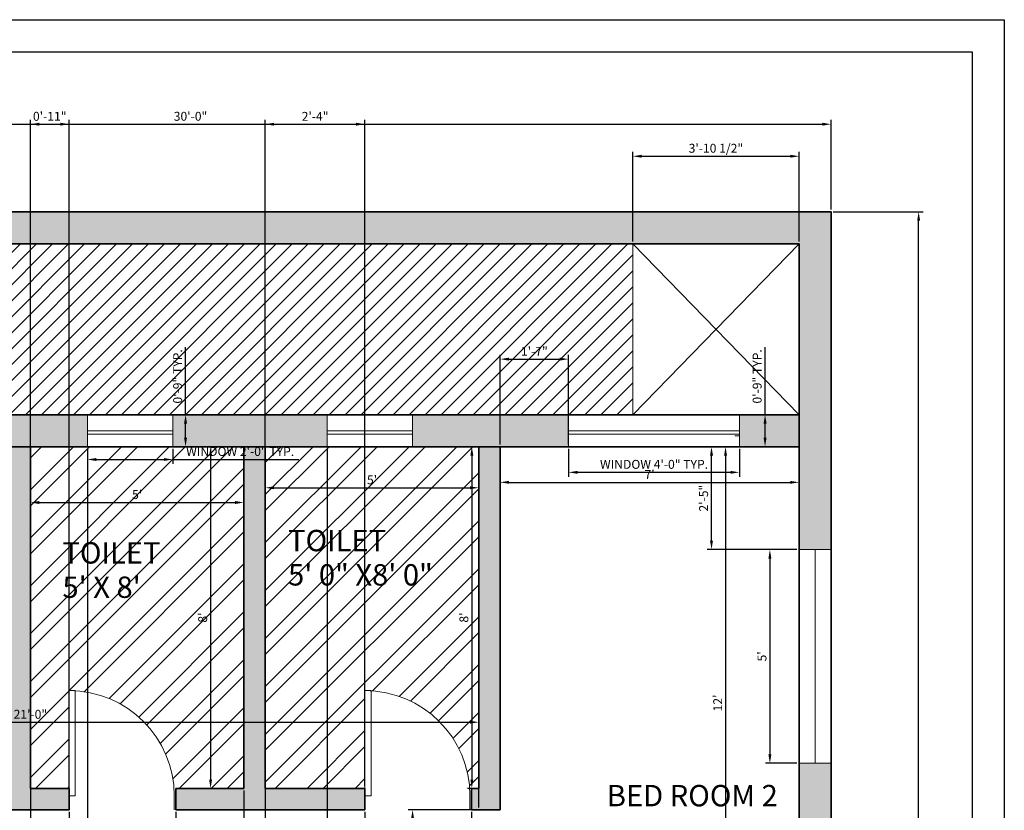
# Model space of a CAD drawing. Units: inches. Extents: x 2998 to 3448, y 1620 to 2377.
# Tile 5 of 5: x 3171 to 3448, y 2155 to 2377. Entities that reach past the tile are written whole.
import ezdxf

# ---------------------------------------------------------------- set-up
doc = ezdxf.new("R2010")
doc.units = ezdxf.units.IN
doc.layers.get('Defpoints').update_dxf_attribs({"color": 110})
for name, color, linetype, lineweight in [('A-ANNO-DIMS', 2, 'Continuous', 18), ('A-ANNO-TTLB', 7, 'Continuous', 25), ('A-AREA-IDEN', 130, 'Continuous', 18), ('A-DOOR', 3, 'Continuous', 18), ('A-FLOR-OPEN', 7, 'Continuous', 18), ('A-FLOR-PATT', 18, 'Continuous', 13), ('A-GLAZ', 4, 'Continuous', 18), ('A-WALL-PATT', 18, 'Continuous', 13), ('C-PROP', 7, 'Continuous', 35), ('L-HRDS-PATT', 175, 'Continuous', 13), ('WALL', 7, 'Continuous', 35)]:
    doc.layers.add(name, color=color, linetype=linetype, lineweight=lineweight)
doc.styles.get("Standard").update_dxf_attribs({"font": 'arial.ttf'})
doc.dimstyles.new('Copy of ISO-25', dxfattribs={"dimtxt": 2.5, "dimasz": 2.5, "dimexe": 1.25, "dimexo": 0.625, "dimtad": 1, "dimdec": 1, "dimlunit": 4, "dimtxsty": 'Standard', "dimcen": 2.5, "dimadec": 0, "dimazin": 0, "dimtfac": 1, "dimtdec": 1, "dimtmove": 0, "dimatfit": 3, "dimfxl": 1, "dimarcsym": 0})

# ---------------------------------------------------------------- blocks, each defined once
blk = doc.blocks.new('*U2')
for p, q in [((0, 0), (0, -100)), ((750, 0), (750, -100))]:
    blk.add_line(p, q)
blk.add_lwpolyline([(0, 0), (0, 750), (43.75, 750), (43.75, 0)], close=True)
blk.add_arc((0, 0), 750, 0, 90)
blk = doc.blocks.new('*D8')
at = {"layer": 'A-ANNO-DIMS', "color": 0, "lineweight": -2, "transparency": 16777216}
for p, q in [((3174.12, 2256.15), (3174.12, 2239.84)), ((3234.12, 2256.15), (3234.12, 2239.84)), ((3176.62, 2241.09), (3231.62, 2241.09))]:
    blk.add_line(p, q, dxfattribs=at)
at = {"layer": 'A-ANNO-DIMS', "color": 0, "transparency": 16777216}
for points in [[(3176.62, 2241.51), (3176.62, 2240.68), (3174.12, 2241.09)], [(3231.62, 2241.51), (3231.62, 2240.68), (3234.12, 2241.09)]]:
    blk.add_solid(points, dxfattribs=at)
at = {"layer": 'Defpoints', "color": 0, "transparency": 16777216}
for p in [(3174.12, 2256.77), (3234.12, 2256.77), (3234.12, 2241.09)]:
    blk.add_point(p, dxfattribs=at)
at = {"layer": 'A-ANNO-DIMS', "color": 0, "transparency": 16777216, "insert": (3204.12, 2242.99), "char_height": 2.5, "attachment_point": 5}
blk.add_mtext("5'", dxfattribs=at)
blk = doc.blocks.new('*D9')
at = {"layer": 'A-ANNO-DIMS', "color": 0, "lineweight": -2, "transparency": 16777216}
for p, q in [((3233.49, 2256.77), (3223.51, 2256.77)), ((3224.76, 2254.27), (3224.76, 2163.27)), ((3233.49, 2160.77), (3223.51, 2160.77))]:
    blk.add_line(p, q, dxfattribs=at)
at = {"layer": 'A-ANNO-DIMS', "color": 0, "transparency": 16777216}
for points in [[(3224.34, 2254.27), (3225.18, 2254.27), (3224.76, 2256.77)], [(3224.34, 2163.27), (3225.18, 2163.27), (3224.76, 2160.77)]]:
    blk.add_solid(points, dxfattribs=at)
at = {"layer": 'Defpoints', "color": 0, "transparency": 16777216}
for p in [(3234.12, 2256.77), (3224.76, 2160.77), (3234.12, 2160.77)]:
    blk.add_point(p, dxfattribs=at)
at = {"layer": 'A-ANNO-DIMS', "color": 0, "transparency": 16777216, "insert": (3222.86, 2208.77), "char_height": 2.5, "attachment_point": 5, "rotation": 90}
blk.add_mtext("8'", dxfattribs=at)
blk = doc.blocks.new('*D10')
at = {"layer": 'A-ANNO-DIMS', "color": 0, "lineweight": -2, "transparency": 16777216}
for p, q in [((3240.12, 2256.15), (3240.12, 2243.98)), ((3300.12, 2256.15), (3300.12, 2243.98)), ((3242.62, 2245.23), (3297.62, 2245.23))]:
    blk.add_line(p, q, dxfattribs=at)
at = {"layer": 'A-ANNO-DIMS', "color": 0, "transparency": 16777216}
for points in [[(3242.62, 2245.65), (3242.62, 2244.82), (3240.12, 2245.23)], [(3297.62, 2245.65), (3297.62, 2244.82), (3300.12, 2245.23)]]:
    blk.add_solid(points, dxfattribs=at)
at = {"layer": 'Defpoints', "color": 0, "transparency": 16777216}
for p in [(3240.12, 2256.77), (3300.12, 2256.77), (3300.12, 2245.23)]:
    blk.add_point(p, dxfattribs=at)
at = {"layer": 'A-ANNO-DIMS', "color": 0, "transparency": 16777216, "insert": (3270.12, 2247.13), "char_height": 2.5, "attachment_point": 5}
blk.add_mtext("5'", dxfattribs=at)
blk = doc.blocks.new('*D11')
at = {"layer": 'A-ANNO-DIMS', "color": 0, "lineweight": -2, "transparency": 16777216}
for p, q in [((3299.49, 2256.77), (3296.92, 2256.77)), ((3298.17, 2254.27), (3298.17, 2163.27)), ((3299.49, 2160.77), (3296.92, 2160.77))]:
    blk.add_line(p, q, dxfattribs=at)
at = {"layer": 'A-ANNO-DIMS', "color": 0, "transparency": 16777216}
for points in [[(3297.75, 2254.27), (3298.58, 2254.27), (3298.17, 2256.77)], [(3297.75, 2163.27), (3298.58, 2163.27), (3298.17, 2160.77)]]:
    blk.add_solid(points, dxfattribs=at)
at = {"layer": 'Defpoints', "color": 0, "transparency": 16777216}
for p in [(3300.12, 2256.77), (3298.17, 2160.77), (3300.12, 2160.77)]:
    blk.add_point(p, dxfattribs=at)
at = {"layer": 'A-ANNO-DIMS', "color": 0, "transparency": 16777216, "insert": (3296.26, 2208.77), "char_height": 2.5, "attachment_point": 5, "rotation": 90}
blk.add_mtext("8'", dxfattribs=at)
blk = doc.blocks.new('*D12')
at = {"layer": 'A-ANNO-DIMS', "color": 0, "lineweight": -2, "transparency": 16777216}
for p, q in [((3306.12, 2256.15), (3306.12, 2245.51)), ((3390.12, 2256.15), (3390.12, 2245.51)), ((3308.62, 2246.76), (3387.62, 2246.76))]:
    blk.add_line(p, q, dxfattribs=at)
at = {"layer": 'A-ANNO-DIMS', "color": 0, "transparency": 16777216}
for points in [[(3308.62, 2247.18), (3308.62, 2246.35), (3306.12, 2246.76)], [(3387.62, 2247.18), (3387.62, 2246.35), (3390.12, 2246.76)]]:
    blk.add_solid(points, dxfattribs=at)
at = {"layer": 'Defpoints', "color": 0, "transparency": 16777216}
for p in [(3306.12, 2256.77), (3390.12, 2256.77), (3390.12, 2246.76)]:
    blk.add_point(p, dxfattribs=at)
at = {"layer": 'A-ANNO-DIMS', "color": 0, "transparency": 16777216, "insert": (3348.12, 2248.64), "char_height": 2.5, "attachment_point": 5}
blk.add_mtext("7'", dxfattribs=at)
blk = doc.blocks.new('*D13')
at = {"layer": 'A-ANNO-DIMS', "color": 0, "lineweight": -2, "transparency": 16777216}
for p, q in [((3389.49, 2256.77), (3368.21, 2256.77)), ((3369.46, 2254.27), (3369.46, 2115.27)), ((3389.49, 2112.77), (3368.21, 2112.77))]:
    blk.add_line(p, q, dxfattribs=at)
at = {"layer": 'A-ANNO-DIMS', "color": 0, "transparency": 16777216}
for points in [[(3369.04, 2254.27), (3369.87, 2254.27), (3369.46, 2256.77)], [(3369.04, 2115.27), (3369.87, 2115.27), (3369.46, 2112.77)]]:
    blk.add_solid(points, dxfattribs=at)
at = {"layer": 'Defpoints', "color": 0, "transparency": 16777216}
for p in [(3390.12, 2256.77), (3369.46, 2112.77), (3390.12, 2112.77)]:
    blk.add_point(p, dxfattribs=at)
at = {"layer": 'A-ANNO-DIMS', "color": 0, "transparency": 16777216, "insert": (3367.58, 2184.77), "char_height": 2.5, "attachment_point": 5, "rotation": 90}
blk.add_mtext("12'", dxfattribs=at)
blk = doc.blocks.new('*D23')
at = {"layer": 'A-ANNO-DIMS', "color": 0, "lineweight": -2, "transparency": 16777216}
for p, q in [((3389.49, 2227.86), (3380.67, 2227.86)), ((3381.92, 2225.36), (3381.92, 2170.36)), ((3389.49, 2167.86), (3380.67, 2167.86))]:
    blk.add_line(p, q, dxfattribs=at)
at = {"layer": 'A-ANNO-DIMS', "color": 0, "transparency": 16777216}
for points in [[(3381.5, 2225.36), (3382.34, 2225.36), (3381.92, 2227.86)], [(3381.5, 2170.36), (3382.34, 2170.36), (3381.92, 2167.86)]]:
    blk.add_solid(points, dxfattribs=at)
at = {"layer": 'Defpoints', "color": 0, "transparency": 16777216}
for p in [(3390.12, 2227.86), (3381.92, 2167.86), (3390.12, 2167.86)]:
    blk.add_point(p, dxfattribs=at)
at = {"layer": 'A-ANNO-DIMS', "color": 0, "transparency": 16777216, "insert": (3380.02, 2197.86), "char_height": 2.5, "attachment_point": 5, "rotation": 90}
blk.add_mtext("5'", dxfattribs=at)
blk = doc.blocks.new('WIN-24IN')
for p, q in [((0, 0), (0, 9)), ((0, 9), (24, 9)), ((24, 9), (24, 0)), ((0, 4.5), (24, 4.5)), ((0, 3.5), (24, 3.5))]:
    blk.add_line(p, q)
blk = doc.blocks.new('WIN-48IN')
for p, q in [((0, 0), (0, 9)), ((0, 9), (48, 9)), ((48, 9), (48, 0)), ((0, 4.5), (48, 4.5)), ((0, 3.5), (48, 3.5))]:
    blk.add_line(p, q)
blk = doc.blocks.new('*D31')
at = {"layer": 'A-ANNO-DIMS', "color": 0, "lineweight": -2, "transparency": 16777216}
for p, q in [((3325.36, 2256.15), (3325.36, 2248.32)), ((3373.36, 2256.15), (3373.36, 2248.32)), ((3327.86, 2249.57), (3370.86, 2249.57))]:
    blk.add_line(p, q, dxfattribs=at)
at = {"layer": 'A-ANNO-DIMS', "color": 0, "transparency": 16777216}
for points in [[(3327.86, 2249.99), (3327.86, 2249.16), (3325.36, 2249.57)], [(3370.86, 2249.99), (3370.86, 2249.16), (3373.36, 2249.57)]]:
    blk.add_solid(points, dxfattribs=at)
at = {"layer": 'Defpoints', "color": 0}
for p in [(3325.36, 2256.77), (3373.36, 2256.77), (3373.36, 2249.57)]:
    blk.add_point(p, dxfattribs=at)
at = {"layer": 'A-ANNO-DIMS', "color": 0, "transparency": 16777216, "insert": (3349.36, 2251.49), "char_height": 2.5, "attachment_point": 5}
blk.add_mtext('WINDOW 4\'-0" TYP.', dxfattribs=at)
blk = doc.blocks.new('*D32')
at = {"layer": 'A-ANNO-DIMS', "color": 0, "lineweight": -2, "transparency": 16777216}
for p, q in [((3380.56, 2265.77), (3380.56, 2284.76)), ((3373.99, 2265.77), (3381.81, 2265.77)), ((3380.56, 2259.27), (3380.56, 2263.27)), ((3373.99, 2256.77), (3381.81, 2256.77))]:
    blk.add_line(p, q, dxfattribs=at)
at = {"layer": 'A-ANNO-DIMS', "color": 0, "transparency": 16777216}
for points in [[(3380.15, 2263.27), (3380.98, 2263.27), (3380.56, 2265.77)], [(3380.15, 2259.27), (3380.98, 2259.27), (3380.56, 2256.77)]]:
    blk.add_solid(points, dxfattribs=at)
at = {"layer": 'Defpoints', "color": 0}
for p in [(3373.36, 2265.77), (3380.56, 2265.77), (3373.36, 2256.77)]:
    blk.add_point(p, dxfattribs=at)
at = {"layer": 'A-ANNO-DIMS', "color": 0, "transparency": 16777216, "insert": (3378.66, 2276.52), "char_height": 2.5, "attachment_point": 5, "rotation": 90}
blk.add_mtext('0\'-9" TYP.', dxfattribs=at)
blk = doc.blocks.new('*D33')
at = {"layer": 'A-ANNO-DIMS', "color": 0, "lineweight": -2, "transparency": 16777216}
for p, q in [((3190.13, 2256.15), (3190.13, 2251.92)), ((3214.13, 2256.15), (3214.13, 2251.92)), ((3192.63, 2253.17), (3211.63, 2253.17)), ((3214.13, 2253.17), (3249.51, 2253.17))]:
    blk.add_line(p, q, dxfattribs=at)
at = {"layer": 'A-ANNO-DIMS', "color": 0, "transparency": 16777216}
for points in [[(3192.63, 2253.59), (3192.63, 2252.76), (3190.13, 2253.17)], [(3211.63, 2253.59), (3211.63, 2252.76), (3214.13, 2253.17)]]:
    blk.add_solid(points, dxfattribs=at)
at = {"layer": 'Defpoints', "color": 0}
for p in [(3190.13, 2256.77), (3214.13, 2256.77), (3214.13, 2253.17)]:
    blk.add_point(p, dxfattribs=at)
at = {"layer": 'A-ANNO-DIMS', "color": 0, "transparency": 16777216, "insert": (3233.07, 2255.09), "char_height": 2.5, "attachment_point": 5}
blk.add_mtext('WINDOW 2\'-0" TYP.', dxfattribs=at)
blk = doc.blocks.new('*D34')
at = {"layer": 'A-ANNO-DIMS', "color": 0, "lineweight": -2, "transparency": 16777216}
for p, q in [((3217.73, 2265.77), (3217.73, 2284.76)), ((3214.75, 2265.77), (3218.98, 2265.77)), ((3217.73, 2259.27), (3217.73, 2263.27)), ((3214.75, 2256.77), (3218.98, 2256.77))]:
    blk.add_line(p, q, dxfattribs=at)
at = {"layer": 'A-ANNO-DIMS', "color": 0, "transparency": 16777216}
for points in [[(3217.31, 2263.27), (3218.14, 2263.27), (3217.73, 2265.77)], [(3217.31, 2259.27), (3218.14, 2259.27), (3217.73, 2256.77)]]:
    blk.add_solid(points, dxfattribs=at)
at = {"layer": 'Defpoints', "color": 0}
for p in [(3214.13, 2265.77), (3217.73, 2265.77), (3214.13, 2256.77)]:
    blk.add_point(p, dxfattribs=at)
at = {"layer": 'A-ANNO-DIMS', "color": 0, "transparency": 16777216, "insert": (3215.83, 2276.52), "char_height": 2.5, "attachment_point": 5, "rotation": 90}
blk.add_mtext('0\'-9" TYP.', dxfattribs=at)
blk = doc.blocks.new('*D39')
at = {"layer": 'A-ANNO-DIMS', "color": 0, "lineweight": -2, "transparency": 16777216}
for p, q in [((3039.12, 2323.4), (3039.12, 2348.62)), ((3041.62, 2347.37), (3396.62, 2347.37)), ((3399.12, 2323.4), (3399.12, 2348.62))]:
    blk.add_line(p, q, dxfattribs=at)
at = {"layer": 'A-ANNO-DIMS', "color": 0, "transparency": 16777216}
for points in [[(3041.62, 2347.79), (3041.62, 2346.96), (3039.12, 2347.37)], [(3396.62, 2347.79), (3396.62, 2346.96), (3399.12, 2347.37)]]:
    blk.add_solid(points, dxfattribs=at)
at = {"layer": 'Defpoints', "color": 0}
for p in [(3399.12, 2347.37), (3039.12, 2322.77), (3399.12, 2322.77)]:
    blk.add_point(p, dxfattribs=at)
at = {"layer": 'A-ANNO-DIMS', "color": 0, "transparency": 16777216, "insert": (3219.12, 2349.27), "char_height": 2.5, "attachment_point": 5}
blk.add_mtext('30\'-0"', dxfattribs=at)
blk = doc.blocks.new('*D40')
at = {"layer": 'A-ANNO-DIMS', "color": 0, "lineweight": -2, "transparency": 16777216}
for p, q in [((3399.74, 2322.77), (3424.97, 2322.77)), ((3423.72, 1845.27), (3423.72, 2320.27)), ((3399.74, 1842.77), (3424.97, 1842.77))]:
    blk.add_line(p, q, dxfattribs=at)
at = {"layer": 'A-ANNO-DIMS', "color": 0, "transparency": 16777216}
for points in [[(3423.3, 2320.27), (3424.14, 2320.27), (3423.72, 2322.77)], [(3423.3, 1845.27), (3424.14, 1845.27), (3423.72, 1842.77)]]:
    blk.add_solid(points, dxfattribs=at)
at = {"layer": 'Defpoints', "color": 0}
for p in [(3399.12, 2322.77), (3423.72, 2322.77), (3399.12, 1842.77)]:
    blk.add_point(p, dxfattribs=at)
at = {"layer": 'A-ANNO-DIMS', "color": 0, "transparency": 16777216, "insert": (3421.82, 2082.77), "char_height": 2.5, "attachment_point": 5, "rotation": 90}
blk.add_mtext('40\'-0"', dxfattribs=at)
blk = doc.blocks.new('*D51')
at = {"layer": 'A-ANNO-DIMS', "color": 0, "lineweight": -2, "transparency": 16777216}
for p, q in [((3174.12, 2256.15), (3174.12, 1816.92)), ((3190.13, 2256.15), (3190.13, 1816.92)), ((3176.62, 1818.17), (3187.63, 1818.17))]:
    blk.add_line(p, q, dxfattribs=at)
at = {"layer": 'A-ANNO-DIMS', "color": 0, "transparency": 16777216}
for points in [[(3176.62, 1818.59), (3176.62, 1817.76), (3174.12, 1818.17)], [(3187.63, 1818.59), (3187.63, 1817.76), (3190.13, 1818.17)]]:
    blk.add_solid(points, dxfattribs=at)
at = {"layer": 'Defpoints', "color": 0}
for p in [(3174.12, 2256.77), (3190.13, 2256.77), (3190.13, 1818.17)]:
    blk.add_point(p, dxfattribs=at)
at = {"layer": 'A-ANNO-DIMS', "color": 0, "transparency": 16777216, "insert": (3182.12, 1820.05), "char_height": 2.5, "attachment_point": 5}
blk.add_mtext('1\'-4"', dxfattribs=at)
blk = doc.blocks.new('*D52')
at = {"layer": 'A-ANNO-DIMS', "color": 0, "lineweight": -2, "transparency": 16777216}
for p, q in [((3240.12, 2256.15), (3240.12, 1816.92)), ((3257.48, 2256.15), (3257.48, 1816.92)), ((3242.62, 1818.17), (3254.98, 1818.17))]:
    blk.add_line(p, q, dxfattribs=at)
at = {"layer": 'A-ANNO-DIMS', "color": 0, "transparency": 16777216}
for points in [[(3242.62, 1818.59), (3242.62, 1817.76), (3240.12, 1818.17)], [(3254.98, 1818.59), (3254.98, 1817.76), (3257.48, 1818.17)]]:
    blk.add_solid(points, dxfattribs=at)
at = {"layer": 'Defpoints', "color": 0}
for p in [(3240.12, 2256.77), (3257.48, 2256.77), (3257.48, 1818.17)]:
    blk.add_point(p, dxfattribs=at)
at = {"layer": 'A-ANNO-DIMS', "color": 0, "transparency": 16777216, "insert": (3248.8, 1820.09), "char_height": 2.5, "attachment_point": 5}
blk.add_mtext('1\'-5 1/2"', dxfattribs=at)
blk = doc.blocks.new('*D53')
at = {"layer": 'A-ANNO-DIMS', "color": 0, "lineweight": -2, "transparency": 16777216}
for p, q in [((3306.12, 2257.4), (3306.12, 2282.62)), ((3325.36, 2257.4), (3325.36, 2282.62)), ((3308.62, 2281.37), (3322.86, 2281.37))]:
    blk.add_line(p, q, dxfattribs=at)
at = {"layer": 'A-ANNO-DIMS', "color": 0, "transparency": 16777216}
for points in [[(3308.62, 2281.79), (3308.62, 2280.96), (3306.12, 2281.37)], [(3322.86, 2281.79), (3322.86, 2280.96), (3325.36, 2281.37)]]:
    blk.add_solid(points, dxfattribs=at)
at = {"layer": 'Defpoints', "color": 0}
for p in [(3325.36, 2281.37), (3306.12, 2256.77), (3325.36, 2256.77)]:
    blk.add_point(p, dxfattribs=at)
at = {"layer": 'A-ANNO-DIMS', "color": 0, "transparency": 16777216, "insert": (3315.74, 2283.25), "char_height": 2.5, "attachment_point": 5}
blk.add_mtext('1\'-7"', dxfattribs=at)
blk = doc.blocks.new('*D54')
at = {"layer": 'A-ANNO-DIMS', "color": 0, "lineweight": -2, "transparency": 16777216}
for p, q in [((3185.01, 2154.15), (3185.01, 1816.92)), ((3215.01, 2154.15), (3215.01, 1816.92)), ((3187.51, 1818.17), (3212.51, 1818.17))]:
    blk.add_line(p, q, dxfattribs=at)
at = {"layer": 'A-ANNO-DIMS', "color": 0, "transparency": 16777216}
for points in [[(3187.51, 1818.59), (3187.51, 1817.76), (3185.01, 1818.17)], [(3212.51, 1818.59), (3212.51, 1817.76), (3215.01, 1818.17)]]:
    blk.add_solid(points, dxfattribs=at)
at = {"layer": 'Defpoints', "color": 0}
for p in [(3185.01, 2154.77), (3215.01, 2154.77), (3215.01, 1818.17)]:
    blk.add_point(p, dxfattribs=at)
at = {"layer": 'A-ANNO-DIMS', "color": 0, "transparency": 16777216, "insert": (3200.01, 1820.07), "char_height": 2.5, "attachment_point": 5}
blk.add_mtext('2\'-6"', dxfattribs=at)
blk = doc.blocks.new('*D55')
at = {"layer": 'A-ANNO-DIMS', "color": 0, "lineweight": -2, "transparency": 16777216}
for p, q in [((3268.12, 2154.15), (3268.12, 1816.92)), ((3298.12, 2154.15), (3298.12, 1816.92)), ((3270.62, 1818.17), (3295.62, 1818.17))]:
    blk.add_line(p, q, dxfattribs=at)
at = {"layer": 'A-ANNO-DIMS', "color": 0, "transparency": 16777216}
for points in [[(3270.62, 1818.59), (3270.62, 1817.76), (3268.12, 1818.17)], [(3295.62, 1818.59), (3295.62, 1817.76), (3298.12, 1818.17)]]:
    blk.add_solid(points, dxfattribs=at)
at = {"layer": 'Defpoints', "color": 0}
for p in [(3268.12, 2154.77), (3298.12, 2154.77), (3298.12, 1818.17)]:
    blk.add_point(p, dxfattribs=at)
at = {"layer": 'A-ANNO-DIMS', "color": 0, "transparency": 16777216, "insert": (3283.12, 1820.07), "char_height": 2.5, "attachment_point": 5}
blk.add_mtext('2\'-6"', dxfattribs=at)
blk = doc.blocks.new('*D56')
at = {"layer": 'A-ANNO-DIMS', "color": 0, "lineweight": -2, "transparency": 16777216}
for p, q in [((3174.12, 2161.4), (3174.12, 2348.62)), ((3176.62, 2347.37), (3182.51, 2347.37)), ((3185.01, 2161.4), (3185.01, 2348.62))]:
    blk.add_line(p, q, dxfattribs=at)
at = {"layer": 'A-ANNO-DIMS', "color": 0, "transparency": 16777216}
for points in [[(3176.62, 2347.79), (3176.62, 2346.96), (3174.12, 2347.37)], [(3182.51, 2347.79), (3182.51, 2346.96), (3185.01, 2347.37)]]:
    blk.add_solid(points, dxfattribs=at)
at = {"layer": 'Defpoints', "color": 0}
for p in [(3185.01, 2347.37), (3174.12, 2160.77), (3185.01, 2160.77)]:
    blk.add_point(p, dxfattribs=at)
at = {"layer": 'A-ANNO-DIMS', "color": 0, "transparency": 16777216, "insert": (3179.56, 2349.27), "char_height": 2.5, "attachment_point": 5}
blk.add_mtext('0\'-11"', dxfattribs=at)
blk = doc.blocks.new('*D57')
at = {"layer": 'A-ANNO-DIMS', "color": 0, "lineweight": -2, "transparency": 16777216}
for p, q in [((3240.12, 2161.4), (3240.12, 2348.62)), ((3242.62, 2347.37), (3265.62, 2347.37)), ((3268.12, 2161.4), (3268.12, 2348.62))]:
    blk.add_line(p, q, dxfattribs=at)
at = {"layer": 'A-ANNO-DIMS', "color": 0, "transparency": 16777216}
for points in [[(3242.62, 2347.79), (3242.62, 2346.96), (3240.12, 2347.37)], [(3265.62, 2347.79), (3265.62, 2346.96), (3268.12, 2347.37)]]:
    blk.add_solid(points, dxfattribs=at)
at = {"layer": 'Defpoints', "color": 0}
for p in [(3268.12, 2347.37), (3240.12, 2160.77), (3268.12, 2160.77)]:
    blk.add_point(p, dxfattribs=at)
at = {"layer": 'A-ANNO-DIMS', "color": 0, "transparency": 16777216, "insert": (3254.12, 2349.25), "char_height": 2.5, "attachment_point": 5}
blk.add_mtext('2\'-4"', dxfattribs=at)
blk = doc.blocks.new('*D58')
at = {"layer": 'A-ANNO-DIMS', "color": 0, "lineweight": -2, "transparency": 16777216}
for p, q in [((3305.49, 2154.77), (3280.27, 2154.77)), ((3281.52, 2121.27), (3281.52, 2152.27)), ((3305.49, 2118.77), (3280.27, 2118.77))]:
    blk.add_line(p, q, dxfattribs=at)
at = {"layer": 'A-ANNO-DIMS', "color": 0, "transparency": 16777216}
for points in [[(3281.1, 2152.27), (3281.94, 2152.27), (3281.52, 2154.77)], [(3281.1, 2121.27), (3281.94, 2121.27), (3281.52, 2118.77)]]:
    blk.add_solid(points, dxfattribs=at)
at = {"layer": 'Defpoints', "color": 0}
for p in [(3281.52, 2154.77), (3306.12, 2154.77), (3306.12, 2118.77)]:
    blk.add_point(p, dxfattribs=at)
at = {"layer": 'A-ANNO-DIMS', "color": 0, "transparency": 16777216, "insert": (3279.62, 2136.77), "char_height": 2.5, "attachment_point": 5, "rotation": 90}
blk.add_mtext('3\'-0"', dxfattribs=at)
blk = doc.blocks.new('*D60')
at = {"layer": 'A-ANNO-DIMS', "color": 0, "lineweight": -2, "transparency": 16777216}
for p, q in [((3048.12, 2155.4), (3048.12, 2180.62)), ((3300.12, 2155.4), (3300.12, 2180.62)), ((3050.62, 2179.37), (3297.62, 2179.37))]:
    blk.add_line(p, q, dxfattribs=at)
at = {"layer": 'A-ANNO-DIMS', "color": 0, "transparency": 16777216}
for points in [[(3050.62, 2179.79), (3050.62, 2178.96), (3048.12, 2179.37)], [(3297.62, 2179.79), (3297.62, 2178.96), (3300.12, 2179.37)]]:
    blk.add_solid(points, dxfattribs=at)
at = {"layer": 'Defpoints', "color": 0}
for p in [(3300.12, 2179.37), (3048.12, 2154.77), (3300.12, 2154.77)]:
    blk.add_point(p, dxfattribs=at)
at = {"layer": 'A-ANNO-DIMS', "color": 0, "transparency": 16777216, "insert": (3174.12, 2181.27), "char_height": 2.5, "attachment_point": 5}
blk.add_mtext('21\'-0"', dxfattribs=at)
blk = doc.blocks.new('*D61')
at = {"layer": 'A-ANNO-DIMS', "color": 0, "lineweight": -2, "transparency": 16777216}
for p, q in [((3389.49, 2256.77), (3364.27, 2256.77)), ((3365.52, 2230.36), (3365.52, 2254.27)), ((3389.49, 2227.86), (3364.27, 2227.86))]:
    blk.add_line(p, q, dxfattribs=at)
at = {"layer": 'A-ANNO-DIMS', "color": 0, "transparency": 16777216}
for points in [[(3365.1, 2254.27), (3365.94, 2254.27), (3365.52, 2256.77)], [(3365.1, 2230.36), (3365.94, 2230.36), (3365.52, 2227.86)]]:
    blk.add_solid(points, dxfattribs=at)
at = {"layer": 'Defpoints', "color": 0}
for p in [(3365.52, 2256.77), (3390.12, 2256.77), (3390.12, 2227.86)]:
    blk.add_point(p, dxfattribs=at)
at = {"layer": 'A-ANNO-DIMS', "color": 0, "transparency": 16777216, "insert": (3363.62, 2242.32), "char_height": 2.5, "attachment_point": 5, "rotation": 90}
blk.add_mtext('2\'-5"', dxfattribs=at)
blk = doc.blocks.new('*D67')
at = {"layer": 'A-ANNO-DIMS', "color": 0, "lineweight": -2, "transparency": 16777216}
for p, q in [((3234.12, 2160.15), (3234.12, 1816.92)), ((3240.12, 2160.15), (3240.12, 1816.92)), ((3231.62, 1818.17), (3229.12, 1818.17)), ((3234.12, 1818.17), (3240.12, 1818.17)), ((3242.62, 1818.17), (3253.01, 1818.17))]:
    blk.add_line(p, q, dxfattribs=at)
at = {"layer": 'A-ANNO-DIMS', "color": 0, "transparency": 16777216}
for points in [[(3231.62, 1818.59), (3231.62, 1817.76), (3234.12, 1818.17)], [(3242.62, 1818.59), (3242.62, 1817.76), (3240.12, 1818.17)]]:
    blk.add_solid(points, dxfattribs=at)
at = {"layer": 'Defpoints', "color": 0}
for p in [(3234.12, 2160.77), (3240.12, 2160.77), (3240.12, 1818.17)]:
    blk.add_point(p, dxfattribs=at)
at = {"layer": 'A-ANNO-DIMS', "color": 0, "transparency": 16777216, "insert": (3249.07, 1820.07), "char_height": 2.5, "attachment_point": 5}
blk.add_mtext('0\'-6"', dxfattribs=at)
blk = doc.blocks.new('*D69')
at = {"layer": 'A-ANNO-DIMS', "color": 0, "lineweight": -2, "transparency": 16777216}
for p, q in [((3343.37, 2314.4), (3343.37, 2339.62)), ((3345.87, 2338.37), (3387.62, 2338.37)), ((3390.12, 2314.4), (3390.12, 2339.62))]:
    blk.add_line(p, q, dxfattribs=at)
at = {"layer": 'A-ANNO-DIMS', "color": 0, "transparency": 16777216}
for points in [[(3345.87, 2338.79), (3345.87, 2337.96), (3343.37, 2338.37)], [(3387.62, 2338.79), (3387.62, 2337.96), (3390.12, 2338.37)]]:
    blk.add_solid(points, dxfattribs=at)
at = {"layer": 'Defpoints', "color": 0}
for p in [(3390.12, 2338.37), (3343.37, 2313.77), (3390.12, 2313.77)]:
    blk.add_point(p, dxfattribs=at)
at = {"layer": 'A-ANNO-DIMS', "color": 0, "transparency": 16777216, "insert": (3366.75, 2340.29), "char_height": 2.5, "attachment_point": 5}
blk.add_mtext('3\'-10 1/2"', dxfattribs=at)

msp = doc.modelspace()

# ---------------------------------------------------------------- hatches: boundary and pattern name
at = {"layer": 'A-FLOR-PATT'}
h = msp.add_hatch(dxfattribs=at)
h.set_pattern_fill('ANSI31', color=256)
h.paths.add_polyline_path([(3264.12, 1950.77), (3252.12, 1950.77), (3252.12, 1955.56), (3250.03, 1955.56), (3250.03, 1991.39, 0.39722), (3216.23, 1955.56), (3216.23, 1950.77), (3204.12, 1950.77), (3204.12, 1890.77), (3216.12, 1890.77), (3216.12, 1881.77), (3252.12, 1881.77), (3252.12, 1890.77), (3264.12, 1890.77)])
h.paths.add_polyline_path([(3343.37, 2313.77), (3048.12, 2313.77), (3048.12, 2265.77), (3059.91, 2265.77), (3059.91, 2296.51), (3061.95, 2296.51), (3061.95, 2296.45, -0.39722), (3094.97, 2261.45), (3095.91, 2265.77), (3343.37, 2265.77)])
h.paths.add_polyline_path([(3220.44, 1918.61), (3261.55, 1918.61), (3261.55, 1927.8), (3220.44, 1927.8)], flags=24)
h.paths.add_polyline_path([(3220.42, 1928.23), (3252.4, 1928.23), (3252.4, 1937.54), (3220.42, 1937.54)], flags=24)
h.paths.add_polyline_path([(3097.58, 2294.93), (3164.02, 2294.93), (3164.02, 2304.23), (3097.58, 2304.23)], flags=24)
h = msp.add_hatch(dxfattribs=at)
h.set_pattern_fill('ANSI32', color=256)
h.paths.add_polyline_path([(3234.12, 2256.77), (3174.12, 2256.77), (3174.12, 2160.77), (3185.01, 2160.77), (3185.01, 2188.24), (3186.73, 2188.24), (3186.73, 2188.19, -0.377118), (3214.46, 2160.77), (3234.12, 2160.77)])
h.paths.add_polyline_path([(3300.12, 2256.77), (3240.12, 2256.77), (3240.12, 2160.77), (3268.12, 2160.77), (3268.12, 2188.24), (3269.84, 2188.24), (3269.84, 2188.19, -0.377118), (3297.57, 2160.77), (3300.12, 2160.77)])
h.paths.add_polyline_path([(3202.2, 2240.4), (3206.06, 2240.4), (3206.06, 2245.55), (3202.2, 2245.55)], flags=24)
h.paths.add_polyline_path([(3225.46, 2206.85), (3225.46, 2210.71), (3220.31, 2210.71), (3220.31, 2206.85)], flags=24)
h.paths.add_polyline_path([(3181.61, 2212.67), (3207.44, 2212.67), (3207.44, 2221.86), (3181.61, 2221.86)], flags=24)
h.paths.add_polyline_path([(3181.59, 2222.28), (3214.03, 2222.28), (3214.03, 2231.6), (3181.59, 2231.6)], flags=24)
h.paths.add_polyline_path([(3268.2, 2244.53), (3272.06, 2244.53), (3272.06, 2249.69), (3268.2, 2249.69)], flags=24)
h.paths.add_polyline_path([(3298.86, 2206.85), (3298.86, 2210.71), (3293.71, 2210.71), (3293.71, 2206.85)], flags=24)
h.paths.add_polyline_path([(3245.01, 2216.14), (3288.45, 2216.14), (3288.45, 2225.33), (3245.01, 2225.33)], flags=24)
h.paths.add_polyline_path([(3244.99, 2225.76), (3277.44, 2225.76), (3277.44, 2235.07), (3244.99, 2235.07)], flags=24)
at = {"layer": 'A-WALL-PATT'}
h = msp.add_hatch(color=256, dxfattribs=at)
h.dxf.hatch_style = 1
h.paths.add_polyline_path([(3399.12, 2322.77), (3039.12, 2322.77), (3039.12, 2132.57), (3048.12, 2132.57), (3048.12, 2154.77), (3048.12, 2313.77), (3390.12, 2313.77), (3390.12, 2227.86), (3399.12, 2227.86)])
h.paths.add_polyline_path([(3048.12, 2072.57), (3039.12, 2072.57), (3039.12, 2041.4), (3048.12, 2041.4)])
h.paths.add_polyline_path([(3399.12, 1997.2), (3390.12, 1997.2), (3390.12, 1851.77), (3274.41, 1851.77), (3274.41, 1842.77), (3399.12, 1842.77)])
h.paths.add_polyline_path([(3195.35, 1851.77), (3048.12, 1851.77), (3048.12, 1857.27), (3048.05, 1858.06), (3047.68, 1858.02), (3047.44, 1857.61), (3047.47, 1857.28), (3047.17, 1857.15), (3047.68, 1858.02), (3045.29, 1857.73), (3045.29, 1842.77), (3195.35, 1842.77)])
h.paths.add_polyline_path([(3399.12, 2167.86), (3390.12, 2167.86), (3390.12, 2112.77), (3390.12, 2103.77), (3390.12, 2045.2), (3399.12, 2045.2)])
h.paths.add_polyline_path([(3390.12, 2112.77), (3306.12, 2112.77), (3306.12, 2118.77), (3304.88, 2118.77), (3300.12, 2118.77), (3300.12, 2112.77), (3300.12, 2103.77), (3390.12, 2103.77)])
h.paths.add_polyline_path([(3257.48, 2265.77), (3214.13, 2265.77), (3214.13, 2256.77), (3257.48, 2256.77)], flags=17)
h.paths.add_polyline_path([(3325.36, 2265.77), (3281.48, 2265.77), (3281.48, 2256.77), (3300.12, 2256.77), (3325.36, 2256.77)], flags=17)
h.paths.add_polyline_path([(3390.12, 2265.77), (3373.36, 2265.77), (3373.36, 2256.77), (3390.12, 2256.77)], flags=17)
h.paths.add_polyline_path([(3190.13, 2265.77), (3155.91, 2265.77), (3155.91, 2256.77), (3190.13, 2256.77)], flags=17)
h.paths.add_polyline_path([(3306.12, 2256.77), (3300.12, 2256.77), (3300.12, 2160.77), (3298.12, 2160.77), (3298.12, 2154.77), (3300.12, 2154.77), (3306.12, 2154.77)], flags=17)
h.paths.add_polyline_path([(3240.12, 2256.77), (3234.12, 2256.77), (3234.12, 2160.77), (3215.01, 2160.77), (3215.01, 2154.77), (3268.12, 2154.77), (3268.12, 2158.71), (3268.12, 2160.77), (3240.12, 2160.77)], flags=17)
h.paths.add_polyline_path([(3174.12, 2256.77), (3168.12, 2256.77), (3168.12, 2160.77), (3138.26, 2160.77), (3138.26, 2154.77), (3174.12, 2154.77), (3185.01, 2154.77), (3185.01, 2158.71), (3185.01, 2160.77), (3174.12, 2160.77)], flags=17)
h.paths.add_polyline_path([(3090.26, 2160.77), (3048.12, 2160.77), (3048.12, 2154.77), (3090.26, 2154.77)], flags=17)
h.paths.add_polyline_path([(3072.12, 2058.77), (3048.12, 2058.77), (3048.12, 2049.77), (3072.12, 2049.77)])
h.paths.add_polyline_path([(3298.3, 1959.77), (3270.12, 1959.77), (3270.12, 2061.77), (3300.12, 2061.77), (3306.12, 2061.77), (3306.12, 2067.77), (3300.12, 2067.77), (3264.12, 2067.77), (3264.12, 2061.77), (3264.12, 1959.77), (3252.12, 1959.77), (3252.12, 1955.56), (3252.12, 1950.77), (3264.12, 1950.77), (3264.12, 1890.77), (3264.12, 1881.77), (3273.12, 1881.77), (3273.12, 1950.77), (3298.3, 1950.77)])
h.paths.add_polyline_path([(3390.12, 1959.77), (3358.3, 1959.77), (3358.3, 1950.77), (3390.12, 1950.77)], flags=17)
h.paths.add_polyline_path([(3216.12, 1959.77), (3154.02, 1959.77), (3154.02, 1950.77), (3216.12, 1950.77)])
h.paths.add_polyline_path([(3204.12, 1950.77), (3195.12, 1950.77), (3195.12, 1890.77), (3195.12, 1881.77), (3216.12, 1881.77), (3216.12, 1890.77), (3204.12, 1890.77)])
h.paths.add_polyline_path([(3094.02, 1959.77), (3048.12, 1959.77), (3048.12, 1950.77), (3094.02, 1950.77)])
h.paths.add_polyline_path([(3045.29, 1981.4), (3040.45, 1981.4), (3040.45, 1842.77), (3045.29, 1842.77), (3045.29, 1857.73)])
h.paths.add_polyline_path([(3059.91, 2261.45), (3059.91, 2265.77), (3048.12, 2265.77), (3048.12, 2256.77), (3059.91, 2256.77)], flags=17)
h.paths.add_polyline_path([(3107.91, 2265.77), (3095.91, 2265.77), (3095.91, 2256.77), (3107.91, 2256.77)], flags=17)
h.paths.add_polyline_path([(3274.41, 1851.77), (3264.12, 1851.77), (3264.12, 1846.71), (3264.12, 1842.77), (3274.41, 1842.77)])
h.paths.add_polyline_path([(3204.35, 1851.77), (3195.35, 1851.77), (3195.35, 1842.77), (3204.35, 1842.77), (3204.35, 1846.71)])
at = {"layer": 'L-HRDS-PATT'}
h = msp.add_hatch(dxfattribs=at)
h.set_pattern_fill('_USER', color=256, pattern_type=0)
h.set_pattern_definition([(0, (0, 0), (0, 1), [])])
h.paths.add_polyline_path([(3195.12, 1950.77), (3154.02, 1950.77), (3154.02, 1914.77), (3084.12, 1914.77), (3084.12, 1881.77), (3195.12, 1881.77), (3195.12, 1890.77)])
h.paths.add_polyline_path([(3107.62, 2003.86), (3160.38, 2003.86), (3160.38, 2013.05), (3107.62, 2013.05)], flags=9)
h.paths.add_polyline_path([(3107.6, 2013.48), (3161.48, 2013.48), (3161.48, 2022.79), (3107.6, 2022.79)], flags=9)
h.paths.add_polyline_path([(3162.21, 2109.19), (3212.64, 2109.19), (3212.64, 2118.38), (3162.21, 2118.38)], flags=9)
h.paths.add_polyline_path([(3162.19, 2118.81), (3194.63, 2118.81), (3194.63, 2128.12), (3162.19, 2128.12)], flags=9)
h.paths.add_polyline_path([(3334.58, 2144.47), (3389.67, 2144.47), (3389.67, 2153.66), (3334.58, 2153.66)], flags=9)
h.paths.add_polyline_path([(3334.56, 2154.09), (3390.29, 2154.09), (3390.29, 2163.4), (3334.56, 2163.4)], flags=9)
h.paths.add_polyline_path([(3245.01, 2216.14), (3288.45, 2216.14), (3288.45, 2225.33), (3245.01, 2225.33)], flags=9)
h.paths.add_polyline_path([(3244.99, 2225.76), (3277.44, 2225.76), (3277.44, 2235.07), (3244.99, 2235.07)], flags=9)
h.paths.add_polyline_path([(3181.61, 2212.67), (3207.44, 2212.67), (3207.44, 2221.86), (3181.61, 2221.86)], flags=9)
h.paths.add_polyline_path([(3181.59, 2222.28), (3214.03, 2222.28), (3214.03, 2231.6), (3181.59, 2231.6)], flags=9)
h.paths.add_polyline_path([(3075.92, 2206.31), (3126.35, 2206.31), (3126.35, 2215.5), (3075.92, 2215.5)], flags=9)
h.paths.add_polyline_path([(3075.9, 2215.93), (3115.79, 2215.93), (3115.79, 2225.24), (3075.9, 2225.24)], flags=9)
h.paths.add_polyline_path([(3097.58, 2294.93), (3164.02, 2294.93), (3164.02, 2304.23), (3097.58, 2304.23)], flags=9)
h = msp.add_hatch(dxfattribs=at)
h.set_pattern_fill('ANGLE', color=256)
h.set_pattern_definition([(0, (0, 0), (0, 6.985), [5.08, -1.905]), (90, (0, 0), (-6.985, 4e-16), [5.08, -1.905])])
h.paths.add_polyline_path([(3390.12, 1950.77), (3358.3, 1950.77), (3273.12, 1950.77), (3273.12, 1881.77), (3268.62, 1881.77), (3268.62, 1851.77), (3390.12, 1851.77)])
h.paths.add_polyline_path([(3334.58, 2144.47), (3389.67, 2144.47), (3389.67, 2153.66), (3334.58, 2153.66)], flags=9)
h.paths.add_polyline_path([(3334.56, 2154.09), (3390.29, 2154.09), (3390.29, 2163.4), (3334.56, 2163.4)], flags=9)
h.paths.add_polyline_path([(3220.44, 1918.61), (3261.55, 1918.61), (3261.55, 1927.8), (3220.44, 1927.8)], flags=9)
h.paths.add_polyline_path([(3220.42, 1928.23), (3252.4, 1928.23), (3252.4, 1937.54), (3220.42, 1937.54)], flags=9)
h.paths.add_polyline_path([(3220.62, 1853.01), (3246.55, 1853.01), (3246.55, 1862.32), (3220.62, 1862.32)], flags=9)
h.paths.add_polyline_path([(3084.85, 1856.81), (3130.62, 1856.81), (3130.62, 1866), (3084.85, 1866)], flags=9)
h.paths.add_polyline_path([(3084.83, 1866.42), (3123.8, 1866.42), (3123.8, 1875.73), (3084.83, 1875.73)], flags=9)
h.paths.add_polyline_path([(3297.1, 1896.73), (3349.87, 1896.73), (3349.87, 1905.92), (3297.1, 1905.92)], flags=24)
h.paths.add_polyline_path([(3297.08, 1906.35), (3357.94, 1906.35), (3357.94, 1915.66), (3297.08, 1915.66)], flags=24)
h.paths.add_polyline_path([(3107.62, 2003.86), (3160.38, 2003.86), (3160.38, 2013.05), (3107.62, 2013.05)], flags=9)
h.paths.add_polyline_path([(3107.6, 2013.48), (3161.48, 2013.48), (3161.48, 2022.79), (3107.6, 2022.79)], flags=9)
h.paths.add_polyline_path([(3294.47, 2015.87), (3347.23, 2015.87), (3347.23, 2025.06), (3294.47, 2025.06)], flags=9)
h.paths.add_polyline_path([(3294.45, 2025.49), (3350.19, 2025.49), (3350.19, 2034.8), (3294.45, 2034.8)], flags=9)
h.paths.add_polyline_path([(3162.21, 2109.19), (3212.64, 2109.19), (3212.64, 2118.38), (3162.21, 2118.38)], flags=9)
h.paths.add_polyline_path([(3162.19, 2118.81), (3194.63, 2118.81), (3194.63, 2128.12), (3162.19, 2128.12)], flags=9)
h.paths.add_polyline_path([(3075.92, 2206.31), (3126.35, 2206.31), (3126.35, 2215.5), (3075.92, 2215.5)], flags=9)
h.paths.add_polyline_path([(3075.9, 2215.93), (3115.79, 2215.93), (3115.79, 2225.24), (3075.9, 2225.24)], flags=9)

# ---------------------------------------------------------------- linework, layer by layer
at = {"layer": 'A-ANNO-TTLB'}
for points in [[(2998.07, 2376.74), (3447.79, 2376.74), (3447.79, 1619.66), (2998.07, 1619.66)], [(3007.07, 2367.74), (3438.79, 2367.74), (3438.79, 1628.66), (3007.07, 1628.66)]]:
    msp.add_lwpolyline(points, close=True, dxfattribs=at)
at = {"layer": 'A-FLOR-OPEN'}
for p, q in [((3390.12, 2313.77), (3343.37, 2313.77)), ((3343.37, 2313.77), (3343.37, 2265.77)), ((3343.37, 2313.77), (3390.12, 2265.77)), ((3343.37, 2265.77), (3390.12, 2313.77)), ((3390.12, 2265.77), (3343.37, 2265.77))]:
    msp.add_line(p, q, dxfattribs=at)
at = {"layer": 'A-GLAZ'}
for p, q in [((3373.36, 2261.27), (3373.36, 2259.87)), ((3373.36, 2259.87), (3372.07, 2259.87)), ((3390.12, 2227.86), (3399.12, 2227.86)), ((3390.12, 2227.86), (3390.12, 2167.86)), ((3394.62, 2227.86), (3394.62, 2167.86)), ((3399.12, 2227.86), (3399.12, 2167.86)), ((3399.12, 2167.86), (3390.12, 2167.86))]:
    msp.add_line(p, q, dxfattribs=at)
at = {"layer": 'C-PROP'}
for points in [[(3039.12, 2322.77), (3399.12, 2322.77), (3399.12, 1842.77), (3039.12, 1842.77)], [(3048.12, 2313.77), (3390.12, 2313.77), (3390.12, 1851.77), (3048.12, 1851.77)]]:
    msp.add_lwpolyline(points, close=True, dxfattribs=at)
at = {"layer": 'WALL'}
for p, q in [((3095.91, 2265.77), (3390.12, 2265.77)), ((3390.12, 2265.77), (3390.12, 2256.77)), ((3390.12, 2256.77), (3095.91, 2256.77)), ((3168.12, 2256.77), (3174.12, 2256.77)), ((3174.12, 2256.77), (3174.12, 2160.77)), ((3174.12, 2256.77), (3234.12, 2256.77)), ((3174.12, 2256.77), (3190.13, 2256.77)), ((3234.12, 2256.77), (3234.12, 2160.77)), ((3240.12, 2160.77), (3240.12, 2256.77)), ((3240.12, 2256.77), (3300.12, 2256.77)), ((3240.12, 2256.77), (3257.48, 2256.77)), ((3300.12, 2256.77), (3300.12, 2160.77)), ((3306.12, 2154.77), (3306.12, 2256.77)), ((3306.12, 2256.77), (3325.36, 2256.77)), ((3390.12, 2256.77), (3390.12, 2112.77)), ((3390.12, 2256.77), (3390.12, 2227.86)), ((3174.12, 2160.77), (3185.01, 2160.77)), ((3174.12, 2160.77), (3185.01, 2160.77)), ((3185.01, 2160.77), (3174.12, 2160.77)), ((3185.01, 2160.77), (3185.01, 2154.77)), ((3234.12, 2160.77), (3215.01, 2160.77)), ((3215.01, 2154.77), (3215.01, 2160.77)), ((3215.01, 2160.77), (3234.12, 2160.77)), ((3240.12, 2160.77), (3268.12, 2160.77)), ((3268.12, 2160.77), (3240.12, 2160.77)), ((3268.12, 2154.77), (3268.12, 2160.77)), ((3300.12, 2160.77), (3298.12, 2160.77)), ((3300.12, 2160.77), (3298.12, 2160.77)), ((3298.12, 2160.77), (3298.12, 2154.77)), ((3298.12, 2160.77), (3300.12, 2160.77)), ((3306.12, 2154.77), (3306.12, 2160.77)), ((3174.12, 2154.77), (3138.26, 2154.77)), ((3174.12, 2154.77), (3185.01, 2154.77)), ((3215.01, 2154.77), (3268.12, 2154.77)), ((3234.12, 2154.77), (3240.12, 2154.77)), ((3298.12, 2154.77), (3300.12, 2154.77)), ((3306.12, 2154.77), (3300.12, 2154.77))]:
    msp.add_line(p, q, dxfattribs=at)

# ---------------------------------------------------------------- block references
at = {"layer": 'A-DOOR', "xscale": 0.0393700787401575, "yscale": 0.0393700787401575, "zscale": 0.0393700787401575}
for p in [(3185.01, 2158.71), (3268.12, 2158.71)]:
    msp.add_blockref('*U2', p, dxfattribs=at)
at = {"layer": 'A-GLAZ'}
for name, p in [('WIN-24IN', (3190.13, 2256.77)), ('WIN-24IN', (3257.48, 2256.77)), ('WIN-48IN', (3325.36, 2256.77))]:
    msp.add_blockref(name, p, dxfattribs=at)

# ---------------------------------------------------------------- texts
at = {"layer": 'A-AREA-IDEN'}
for s, p in [('TOILET', (3246.54, 2227.41)), ('TOILET', (3183.14, 2223.94)), ('5\' 0" X8\' 0"', (3246.54, 2217.77)), ("5' X 8'", (3183.14, 2214.3)), ('BED ROOM 2', (3336.11, 2155.74))]:
    msp.add_text(s, height=6, dxfattribs=at).set_placement(p)

# ---------------------------------------------------------------- dimensions: what is measured, and where the dimension line sits
at = {"layer": 'A-ANNO-DIMS'}
for base, p1, p2, override, picture, middle in [((3399.12, 2347.37), (3039.12, 2322.77), (3399.12, 2322.77), {"dimdec": 1, "dimlfac": 1, "dimrnd": 0, "dimzin": 1, "dimdsep": 46, "dimlunit": 4, "dimfrac": 2}, '*D39', (3219.12, 2349.27)), ((3185.01, 2347.37), (3174.12, 2160.77), (3185.01, 2160.77), {"dimdec": 1, "dimlfac": 1, "dimrnd": 0, "dimzin": 1, "dimdsep": 46, "dimlunit": 4, "dimfrac": 2}, '*D56', (3179.56, 2349.27)), ((3268.12, 2347.37), (3240.12, 2160.77), (3268.12, 2160.77), {"dimdec": 1, "dimlfac": 1, "dimrnd": 0, "dimzin": 1, "dimdsep": 46, "dimlunit": 4, "dimfrac": 2}, '*D57', (3254.12, 2349.25)), ((3390.1191, 2338.3719), (3343.3727, 2313.7719), (3390.1191, 2313.7719), {"dimdec": 1, "dimlfac": 1, "dimrnd": 0, "dimzin": 1, "dimdsep": 46, "dimlunit": 4, "dimfrac": 2}, '*D69', (3366.7459, 2340.2904)), ((3325.36, 2281.37), (3306.12, 2256.77), (3325.36, 2256.77), {"dimdec": 1, "dimlfac": 1, "dimrnd": 0, "dimzin": 1, "dimdsep": 46, "dimlunit": 4, "dimfrac": 2}, '*D53', (3315.74, 2283.25)), ((3234.12, 2241.09), (3174.12, 2256.77), (3234.12, 2256.77), {"dimclrd": 0, "dimclre": 0, "dimclrt": 0}, '*D8', (3204.12, 2242.99)), ((3190.13, 1818.17), (3174.12, 2256.77), (3190.13, 2256.77), {"dimdec": 1, "dimlfac": 1, "dimrnd": 0, "dimzin": 1, "dimdsep": 46, "dimlunit": 4, "dimfrac": 2}, '*D51', (3182.12, 1820.05)), ((3300.12, 2245.23), (3240.12, 2256.77), (3300.12, 2256.77), {"dimclrd": 0, "dimclre": 0, "dimclrt": 0}, '*D10', (3270.12, 2247.13)), ((3257.48, 1818.17), (3240.12, 2256.77), (3257.48, 2256.77), {"dimdec": 1, "dimlfac": 1, "dimrnd": 0, "dimzin": 1, "dimdsep": 46, "dimlunit": 4, "dimfrac": 2}, '*D52', (3248.8, 1820.09)), ((3390.12, 2246.76), (3306.12, 2256.77), (3390.12, 2256.77), {"dimclrd": 0, "dimclre": 0, "dimclrt": 0}, '*D12', (3348.12, 2248.64)), ((3240.12, 1818.17), (3234.12, 2160.77), (3240.12, 2160.77), {"dimdec": 1, "dimlfac": 1, "dimrnd": 0, "dimzin": 1, "dimdsep": 46, "dimlunit": 4, "dimfrac": 2}, '*D67', (3249.07, 1820.07)), ((3215.01, 1818.17), (3185.01, 2154.77), (3215.01, 2154.77), {"dimdec": 1, "dimlfac": 1, "dimrnd": 0, "dimzin": 1, "dimdsep": 46, "dimlunit": 4, "dimfrac": 2}, '*D54', (3200.01, 1820.07)), ((3298.12, 1818.17), (3268.12, 2154.77), (3298.12, 2154.77), {"dimdec": 1, "dimlfac": 1, "dimrnd": 0, "dimzin": 1, "dimdsep": 46, "dimlunit": 4, "dimfrac": 2}, '*D55', (3283.12, 1820.07))]:
    dim = msp.add_linear_dim(base=base, p1=p1, p2=p2, dimstyle='Copy of ISO-25', override=override, dxfattribs=at)
    dim.commit()
    dim.dimension.update_dxf_attribs({"geometry": picture, "text_midpoint": middle})
for base, p1, p2, angle, override, picture, middle in [((3423.72, 2322.77), (3399.12, 1842.77), (3399.12, 2322.77), 90, {"dimdec": 1, "dimlfac": 1, "dimrnd": 0, "dimzin": 1, "dimdsep": 46, "dimlunit": 4, "dimfrac": 2}, '*D40', (3421.82, 2082.77)), ((3224.76, 2160.77), (3234.12, 2256.77), (3234.12, 2160.77), 90, {"dimclrd": 0, "dimclre": 0, "dimclrt": 0}, '*D9', (3222.86, 2208.77)), ((3298.17, 2160.77), (3300.12, 2256.77), (3300.12, 2160.77), 90, {"dimclrd": 0, "dimclre": 0, "dimclrt": 0}, '*D11', (3296.26, 2208.77)), ((3365.52, 2256.77), (3390.12, 2227.86), (3390.12, 2256.77), 90, {"dimdec": 1, "dimlfac": 1, "dimrnd": 0, "dimzin": 1, "dimdsep": 46, "dimlunit": 4, "dimfrac": 2}, '*D61', (3363.62, 2242.32)), ((3369.46, 2112.77), (3390.12, 2256.77), (3390.12, 2112.77), 90, {"dimclrd": 0, "dimclre": 0, "dimclrt": 0}, '*D13', (3367.58, 2184.77)), ((3381.92, 2167.86), (3390.12, 2227.86), (3390.12, 2167.86), 90, {"dimclrd": 0, "dimclre": 0, "dimclrt": 0}, '*D23', (3380.02, 2197.86)), ((3300.12, 2179.37), (3048.12, 2154.77), (3300.12, 2154.77), 0, {"dimdec": 1, "dimlfac": 1, "dimrnd": 0, "dimzin": 1, "dimdsep": 46, "dimlunit": 4, "dimfrac": 2}, '*D60', (3174.12, 2181.27)), ((3281.52, 2154.77), (3306.12, 2118.77), (3306.12, 2154.77), 90, {"dimdec": 1, "dimlfac": 1, "dimrnd": 0, "dimzin": 1, "dimdsep": 46, "dimlunit": 4, "dimfrac": 2}, '*D58', (3279.62, 2136.77))]:
    dim = msp.add_linear_dim(base=base, p1=p1, p2=p2, angle=angle, dimstyle='Copy of ISO-25', override=override, dxfattribs=at)
    dim.commit()
    dim.dimension.update_dxf_attribs({"geometry": picture, "text_midpoint": middle})
for base, p1, p2, picture, middle in [((3217.73, 2265.77), (3214.13, 2256.77), (3214.13, 2265.77), '*D34', (3215.83, 2276.52)), ((3380.56, 2265.77), (3373.36, 2256.77), (3373.36, 2265.77), '*D32', (3378.66, 2276.52))]:
    dim = msp.add_linear_dim(base=base, p1=p1, p2=p2, angle=90, text='<> TYP.', dimstyle='Copy of ISO-25', override={"dimdec": 1, "dimlfac": 1, "dimrnd": 0, "dimzin": 1, "dimdsep": 46, "dimlunit": 4, "dimfrac": 2}, dxfattribs=at)
    dim.commit()
    dim.dimension.update_dxf_attribs({"geometry": picture, "text_midpoint": middle})
for base, p1, p2, picture, middle in [((3214.13, 2253.17), (3190.13, 2256.77), (3214.13, 2256.77), '*D33', (3233.07, 2255.09)), ((3373.36, 2249.57), (3325.36, 2256.77), (3373.36, 2256.77), '*D31', (3349.36, 2251.49))]:
    dim = msp.add_linear_dim(base=base, p1=p1, p2=p2, text='WINDOW <> TYP.', dimstyle='Copy of ISO-25', override={"dimdec": 1, "dimlfac": 1, "dimrnd": 0, "dimzin": 1, "dimdsep": 46, "dimlunit": 4, "dimfrac": 2}, dxfattribs=at)
    dim.commit()
    dim.dimension.update_dxf_attribs({"geometry": picture, "text_midpoint": middle})

doc.saveas('drawing.dxf')
